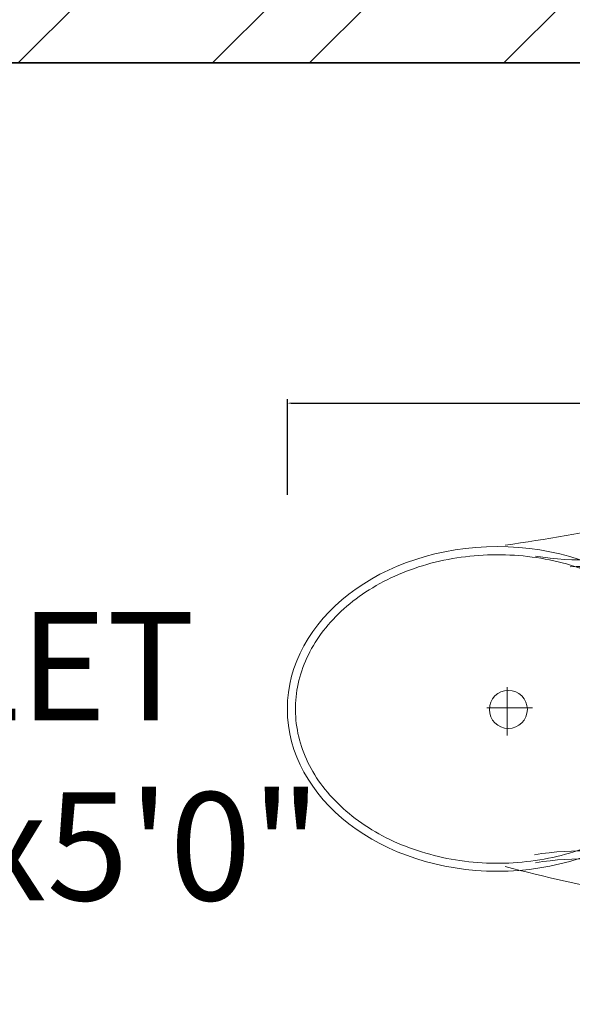
# Model space of a CAD drawing. Units: inches. Extents: x 2168 to 3056, y 1130 to 2629.
# Tile 36 of 42: x 2818 to 2843, y 2217 to 2263. Entities that reach past the tile are written whole.
import ezdxf

# ---------------------------------------------------------------- set-up
doc = ezdxf.new("R2010")
doc.units = ezdxf.units.IN
for name, color, linetype, lineweight in [('A-ANNO-DIMS', 2, 'Continuous', 18), ('A-AREA-IDEN', 7, 'Continuous', 18), ('A-FLOR-FIXT', 9, 'Continuous', 18), ('A-WALL', 7, 'Continuous', 35)]:
    doc.layers.add(name, color=color, linetype=linetype, lineweight=lineweight)
doc.layers.add('A-WALL-PATT', color=143, linetype='Continuous', lineweight=13, true_color=0x7aafdf)
doc.styles.get("Standard").update_dxf_attribs({"font": 'arial.ttf'})
doc.dimstyles.get("Standard").update_dxf_attribs({"dimtxt": 0.18, "dimasz": 0.18, "dimexe": 0.18, "dimexo": 0.0625, "dimgap": 0.09, "dimtad": 0, "dimtih": 1, "dimtoh": 1, "dimdec": 4, "dimzin": 0, "dimdsep": 46, "dimtxsty": 'Standard', "dimcen": 0.09, "dimadec": 0, "dimazin": 0, "dimtfac": 1, "dimtdec": 4, "dimtofl": 0, "dimtmove": 0, "dimatfit": 3, "dimfxl": 1, "dimtolj": 1, "dimtzin": 0, "dimarcsym": 0})

# ---------------------------------------------------------------- blocks, each defined once
blk = doc.blocks.new('A$C31115884')
for p, q in [((257.5, 466.4), (257.5, 523.2)), ((283.1, 497.7), (223.4, 497.7)), ((0, 200), (0, 0)), ((520, 200), (0, 200)), ((520, 0), (520, 200)), ((10, 190), (10, 10)), ((510, 190), (10, 190)), ((510, 10), (510, 190)), ((510, 54.5), (0, 54.5)), ((10, 10), (510, 10)), ((0, 0), (520, 0))]:
    blk.add_line(p, q)
blk.add_circle((255.6, 496.4), 23.6)
for centre, radius, start, end in [((2777.7, -204.6), 2807, 165.4549, 171.7133), ((3237, 905), 2807, 188.2867, 194.5451), ((-294.5, 403.3), 364.7, 324.2091, 9.3499), ((-294.5, 403.3), 374.7, 324.2091, 9.3499), ((805.8, 403.3), 364.7, 170.6501, 215.7909), ((139.5, 406.2), 293.5, 315.8436, 2.6563), ((805.8, 403.3), 374.7, 179.2036, 215.7909), ((383.6, 406.2), 293.5, 190.2774, 224.1564)]:
    blk.add_arc(centre, radius, start, end)
blk.add_ellipse((256.2, 509.9), major_axis=(0, -260.7), ratio=0.772727)
blk.add_open_spline([(256.2, 259.2), (263.1, 259.2), (270, 259.7), (287.8, 262.3), (298.7, 265.1), (319.9, 273.1), (330.2, 278.4), (350.1, 291.1), (359.7, 298.7), (377.7, 315.9), (386.2, 325.5), (401.7, 346.6), (408.8, 358.1), (421.3, 382.5), (426.8, 395.5), (435.9, 422.4), (439.5, 436.4), (444.8, 465.1), (446.5, 479.7), (447.9, 509.2), (447.6, 524), (445, 553.3), (442.7, 567.8), (436.3, 596), (432.1, 609.7), (421.9, 636), (416, 648.6), (402.5, 672.1), (395, 683), (378.6, 703), (369.8, 712.1), (351.1, 728), (341.3, 734.8), (320.9, 746.2), (310.4, 750.7), (288.9, 757.3), (278, 759.4), (256, 761), (245, 760.6), (223.1, 757.2), (212.3, 754.3), (191.1, 746.1), (180.8, 740.7), (160.9, 727.8), (151.4, 720.1), (133.5, 702.7), (125.1, 693), (109.6, 671.7), (102.6, 660.2), (90.2, 635.7), (84.9, 622.7), (76, 595.6), (72.4, 581.6), (67.2, 552.9), (65.6, 538.2), (64.4, 508.8), (64.8, 494), (67.5, 464.7), (69.9, 450.2), (76.6, 422), (80.8, 408.3), (91.1, 382.2), (97.2, 369.7), (110.8, 346.3), (118.4, 335.4), (134.8, 315.6), (143.7, 306.7), (162.4, 290.9), (172.3, 284.2), (192.8, 273), (203.3, 268.6), (224.8, 262.2), (235.8, 260.2), (249.9, 259.3), (253, 259.2), (256.2, 259.2)], degree=3, knots=[0, 0, 0, 0, 0.110105, 0.110105, 0.285049, 0.285049, 0.459994, 0.459994, 0.634938, 0.634938, 0.809882, 0.809882, 0.984827, 0.984827, 1.159771, 1.159771, 1.334715, 1.334715, 1.50966, 1.50966, 1.684604, 1.684604, 1.859549, 1.859549, 2.034493, 2.034493, 2.209437, 2.209437, 2.384382, 2.384382, 2.559326, 2.559326, 2.73427, 2.73427, 2.909215, 2.909215, 3.084159, 3.084159, 3.259103, 3.259103, 3.434048, 3.434048, 3.608992, 3.608992, 3.783936, 3.783936, 3.958881, 3.958881, 4.133825, 4.133825, 4.30877, 4.30877, 4.483714, 4.483714, 4.658658, 4.658658, 4.833603, 4.833603, 5.008547, 5.008547, 5.183491, 5.183491, 5.358436, 5.358436, 5.53338, 5.53338, 5.708324, 5.708324, 5.883269, 5.883269, 6.058213, 6.058213, 6.233158, 6.233158, 6.283185, 6.283185, 6.283185, 6.283185])
blk = doc.blocks.new('*D20')
at = {"layer": 'A-ANNO-DIMS', "color": 0, "lineweight": -2, "transparency": 16777216}
for p, q in [((2830.107, 2240.907), (2830.107, 2245.333)), ((2830.287, 2245.153), (2843.691, 2245.153)), ((2858.647, 2245.153), (2845.243, 2245.153)), ((2858.827, 2240.907), (2858.827, 2245.333))]:
    blk.add_line(p, q, dxfattribs=at)
at = {"layer": 'A-ANNO-DIMS', "color": 0, "transparency": 16777216}
for points in [[(2830.287, 2245.183), (2830.287, 2245.123), (2830.107, 2245.153)], [(2858.647, 2245.183), (2858.647, 2245.123), (2858.827, 2245.153)]]:
    blk.add_solid(points, dxfattribs=at)
at = {"layer": 'Defpoints', "color": 0, "transparency": 16777216}
for p in [(2830.107, 2245.153), (2830.107, 2240.845), (2858.827, 2240.845)]:
    blk.add_point(p, dxfattribs=at)
at = {"layer": 'A-ANNO-DIMS', "color": 0, "transparency": 16777216, "insert": (2844.467, 2245.153), "char_height": 0.18, "attachment_point": 5}
blk.add_mtext('\\A1;WC 29 TYP.', dxfattribs=at)

msp = doc.modelspace()

# ---------------------------------------------------------------- hatches: boundary and pattern name
at = {"layer": 'A-WALL-PATT'}
h = msp.add_hatch(dxfattribs=at)
h.set_pattern_fill('ANSI32', color=256)
h.paths.add_polyline_path([(2463.796, 2409.389), (2467.387, 2409.389), (2467.387, 2413.889), (2454.768, 2413.889), (2454.768, 2411.639), (2454.768, 2409.389), (2459.296, 2409.389), (2459.296, 2265.389), (2455.644, 2265.389), (2455.644, 2260.889), (2467.349, 2260.889), (2467.349, 2263.139), (2467.349, 2265.389), (2463.796, 2265.389)])
h.paths.add_polyline_path([(2431.596, 2413.889), (2409.647, 2413.889), (2409.647, 2409.389), (2431.596, 2409.389), (2431.596, 2411.639)])
h.paths.add_polyline_path([(2349.647, 2413.889), (2331.796, 2413.889), (2331.796, 2362.671), (2336.296, 2362.671), (2336.296, 2409.389), (2349.647, 2409.389), (2349.647, 2411.639)])
h.paths.add_polyline_path([(2634.149, 2411.639), (2634.149, 2413.889), (2562.293, 2413.889), (2562.293, 2409.389), (2595.796, 2409.389), (2595.796, 2280.309), (2595.826, 2280.309), (2595.826, 2265.389), (2499.91, 2265.389), (2499.91, 2260.889), (2550.796, 2260.889), (2550.796, 2117.308), (2555.296, 2117.308), (2555.296, 2168.08), (2571.93, 2168.08), (2571.93, 2176.889), (2559.796, 2176.889), (2559.796, 2256.389), (2640.796, 2256.389), (2640.796, 2176.889), (2626.428, 2176.889), (2626.428, 2168.08), (2645.296, 2168.08), (2645.296, 2116.637), (2649.796, 2116.637), (2649.796, 2260.889), (2691.251, 2260.889), (2691.251, 2263.139), (2691.251, 2265.389), (2670.655, 2265.389), (2670.655, 2265.365), (2600.296, 2265.365), (2600.296, 2280.258), (2600.296, 2409.389), (2634.149, 2409.389)])
h.paths.add_polyline_path([(2600.296, 2473.889), (2612.84, 2473.889), (2612.84, 2478.389), (2572.636, 2478.389), (2572.636, 2473.889), (2595.796, 2473.889), (2595.796, 2413.889), (2600.296, 2413.889)])
h.paths.add_polyline_path([(2535.796, 2473.889), (2548.636, 2473.889), (2548.636, 2478.389), (2531.396, 2478.389), (2531.396, 2413.889), (2521.6, 2413.889), (2521.6, 2409.389), (2539.239, 2409.389), (2539.239, 2411.639), (2539.239, 2413.889), (2535.796, 2413.889)])
h.paths.add_polyline_path([(2664.796, 2478.389), (2636.84, 2478.389), (2636.84, 2473.889), (2660.296, 2473.889), (2660.296, 2413.889), (2656.165, 2413.889), (2656.165, 2409.389), (2671.684, 2409.389), (2671.684, 2411.639), (2671.684, 2413.889), (2664.796, 2413.889)])
h.paths.add_polyline_path([(2705.942, 2413.889), (2695.684, 2413.889), (2695.684, 2409.389), (2705.942, 2409.389)])
h.paths.add_polyline_path([(2741.35, 2413.889), (2728.733, 2413.889), (2728.733, 2411.639), (2728.733, 2409.389), (2732.296, 2409.389), (2732.296, 2265.389), (2725.733, 2265.389), (2725.733, 2260.889), (2740.917, 2260.889), (2740.917, 2263.139), (2740.917, 2265.389), (2736.796, 2265.389), (2736.796, 2409.389), (2741.35, 2409.389)])
h.paths.add_polyline_path([(2785.655, 2413.889), (2764.546, 2413.889), (2764.486, 2409.389), (2785.655, 2409.389), (2785.655, 2411.639)])
h.paths.add_polyline_path([(2864.296, 2413.889), (2845.655, 2413.889), (2845.655, 2409.389), (2859.796, 2409.389), (2859.796, 2368.425), (2864.296, 2368.425)])
h.paths.add_polyline_path([(2864.296, 2308.425), (2862.046, 2308.425), (2859.796, 2308.425), (2859.796, 2265.389), (2774.483, 2265.389), (2774.483, 2263.139), (2774.483, 2260.889), (2781.796, 2260.889), (2781.796, 2226.654), (2786.296, 2226.654), (2786.296, 2260.889), (2859.796, 2260.889), (2859.796, 2241.352), (2864.296, 2241.352)])
h.paths.add_polyline_path([(2864.296, 2217.352), (2862.046, 2217.352), (2859.796, 2217.352), (2859.796, 2200.889), (2786.296, 2200.889), (2786.296, 2205.931), (2784.046, 2205.931), (2781.796, 2205.931), (2781.796, 2150.974), (2786.296, 2150.974), (2786.296, 2161.889), (2859.796, 2161.889), (2859.796, 2144.419), (2864.296, 2144.419)])
h.paths.add_polyline_path([(2859.796, 2196.389), (2859.796, 2166.389), (2786.296, 2166.389), (2786.296, 2196.389)], flags=16)
h.paths.add_polyline_path([(2864.296, 2108.419), (2862.046, 2108.419), (2859.796, 2108.419), (2859.796, 2080.889), (2786.296, 2080.889), (2786.296, 2111.993), (2781.796, 2111.993), (2781.796, 2080.889), (2649.796, 2080.889), (2649.796, 2086.036), (2647.546, 2086.036), (2645.296, 2086.036), (2645.296, 2071.739), (2649.796, 2071.739), (2649.796, 2076.389), (2781.796, 2076.389), (2781.796, 2041.792), (2786.296, 2041.792), (2786.296, 2076.389), (2859.796, 2076.389), (2859.796, 2058.577), (2864.296, 2058.577)])
h.paths.add_polyline_path([(2864.296, 2022.577), (2859.796, 2022.577), (2859.796, 1992.389), (2786.296, 1992.389), (2786.296, 1999.573), (2781.796, 1999.573), (2781.796, 1848.085), (2784.046, 1848.085), (2786.296, 1848.085), (2786.296, 1851.389), (2859.796, 1851.389), (2859.796, 1838.258), (2864.296, 1838.258)], flags=17)
h.paths.add_polyline_path([(2859.796, 1987.889), (2859.796, 1855.889), (2786.296, 1855.889), (2786.296, 1987.889)], flags=16)
h.paths.add_polyline_path([(2823.046, 1987.889), (2841.421, 1921.889), (2823.046, 1855.889)], flags=0)
h.paths.add_polyline_path([(2864.296, 1814.258), (2859.796, 1814.258), (2859.796, 1791.389), (2786.296, 1791.389), (2786.296, 1825.658), (2784.046, 1825.658), (2781.796, 1825.658), (2781.796, 1791.389), (2720.155, 1791.389), (2720.155, 1791.265), (2649.796, 1791.265), (2649.796, 1806.159), (2649.796, 2038.983), (2647.546, 2038.983), (2645.296, 2038.983), (2645.296, 1783.925), (2649.796, 1783.925), (2649.796, 1786.889), (2781.796, 1786.889), (2781.796, 1746.789), (2786.296, 1746.789), (2786.296, 1786.889), (2859.796, 1786.889), (2859.796, 1770.083), (2864.296, 1770.083)])
h.paths.add_polyline_path([(2864.296, 1734.083), (2862.046, 1734.083), (2859.796, 1734.083), (2859.796, 1705.889), (2786.296, 1705.889), (2786.296, 1714.166), (2781.796, 1714.166), (2781.796, 1660.527), (2786.296, 1660.527), (2786.296, 1666.889), (2859.796, 1666.889), (2859.796, 1648.342), (2864.296, 1648.342)])
h.paths.add_polyline_path([(2786.296, 1701.389), (2859.796, 1701.389), (2859.796, 1671.389), (2786.296, 1671.389)], flags=16)
h.paths.add_polyline_path([(2649.796, 1756.576), (2647.546, 1756.576), (2645.296, 1756.576), (2645.296, 1606.889), (2555.296, 1606.889), (2555.296, 1749.513), (2553.046, 1749.513), (2550.796, 1749.513), (2550.796, 1606.889), (2503.006, 1606.889), (2503.006, 1604.639), (2503.006, 1602.389), (2595.796, 1602.389), (2595.849, 1602.389), (2595.849, 1587.495), (2595.796, 1458.389), (2561.502, 1458.389), (2561.502, 1456.139), (2561.502, 1453.889), (2595.796, 1453.889), (2595.796, 1381.889), (2573.438, 1381.889), (2573.438, 1377.389), (2613.01, 1377.389), (2613.01, 1379.639), (2613.01, 1381.889), (2600.296, 1381.889), (2600.296, 1453.889), (2634.327, 1453.889), (2634.327, 1458.389), (2600.296, 1458.389), (2600.296, 1602.389), (2670.655, 1602.389), (2694.095, 1602.389), (2694.095, 1606.889), (2649.796, 1606.889)])
h.paths.add_polyline_path([(2736.796, 1602.389), (2741.562, 1602.389), (2741.562, 1606.889), (2726.203, 1606.889), (2726.203, 1604.639), (2726.203, 1602.389), (2732.296, 1602.389), (2732.296, 1458.389), (2727.899, 1458.389), (2727.899, 1453.889), (2740.821, 1453.889), (2740.821, 1456.139), (2740.821, 1458.389), (2736.796, 1458.389)])
h.paths.add_polyline_path([(2859.796, 1606.889), (2786.296, 1606.889), (2786.296, 1637.334), (2784.046, 1637.334), (2781.796, 1637.334), (2781.796, 1606.889), (2775.612, 1606.889), (2775.612, 1602.389), (2859.796, 1602.389)])
h.paths.add_polyline_path([(2864.296, 1624.342), (2862.046, 1624.342), (2859.796, 1624.342), (2859.796, 1570.39), (2864.296, 1570.39)])
h.paths.add_polyline_path([(2864.296, 1510.39), (2862.046, 1510.39), (2859.796, 1510.39), (2859.796, 1458.389), (2846.735, 1458.389), (2846.735, 1456.139), (2846.735, 1453.889), (2864.296, 1453.889)])
h.paths.add_polyline_path([(2786.735, 1458.389), (2765.444, 1458.389), (2765.444, 1453.889), (2786.735, 1453.889)])
h.paths.add_polyline_path([(2706.004, 1458.389), (2695.36, 1458.389), (2695.36, 1453.889), (2706.004, 1453.889), (2706.004, 1456.139)])
h.paths.add_polyline_path([(2671.36, 1456.139), (2671.36, 1458.389), (2655.986, 1458.389), (2655.986, 1456.139), (2655.986, 1453.889), (2660.296, 1453.889), (2660.296, 1381.889), (2637.01, 1381.889), (2637.01, 1377.389), (2664.796, 1377.389), (2664.796, 1453.889), (2671.36, 1453.889)], flags=17)
h.paths.add_polyline_path([(2539.829, 1458.389), (2520.237, 1458.389), (2520.237, 1453.889), (2531.296, 1453.889), (2531.296, 1377.389), (2546.449, 1377.389), (2546.449, 1379.639), (2546.449, 1381.889), (2535.796, 1381.889), (2535.796, 1453.889), (2539.829, 1453.889)], flags=17)
h.paths.add_polyline_path([(2496.237, 1458.389), (2489.13, 1458.389), (2489.13, 1453.889), (2496.237, 1453.889), (2496.237, 1456.139)])
h.paths.add_polyline_path([(2467.433, 1456.139), (2467.433, 1458.389), (2463.796, 1458.389), (2463.796, 1602.389), (2468.242, 1602.389), (2468.242, 1605.7), (2468.242, 1606.889), (2454.602, 1606.889), (2454.602, 1602.389), (2459.296, 1602.389), (2459.296, 1458.389), (2454.24, 1458.389), (2454.24, 1453.889), (2467.433, 1453.889)])
h.paths.add_polyline_path([(2431.601, 1456.139), (2431.601, 1458.389), (2411.386, 1458.389), (2411.386, 1453.889), (2431.601, 1453.889)])
h.paths.add_polyline_path([(2351.386, 1458.389), (2336.296, 1458.389), (2336.296, 1490.693), (2334.046, 1490.693), (2331.796, 1490.693), (2331.796, 1453.889), (2351.386, 1453.889), (2351.386, 1456.139)])
h.paths.add_polyline_path([(2336.296, 1629.705), (2331.796, 1629.705), (2331.796, 1552.317), (2336.296, 1552.317), (2336.296, 1602.389), (2406.655, 1602.389), (2423.472, 1602.389), (2423.472, 1606.889), (2418.796, 1606.889), (2418.796, 1643.678), (2416.546, 1643.678), (2414.296, 1643.678), (2414.296, 1606.889), (2336.296, 1606.889)])
h.paths.add_polyline_path([(2418.796, 1714.384), (2414.296, 1714.384), (2414.296, 1705.889), (2336.296, 1705.889), (2336.296, 1731.324), (2334.046, 1731.324), (2331.796, 1731.324), (2331.796, 1653.705), (2334.046, 1653.705), (2336.296, 1653.705), (2336.296, 1666.889), (2414.296, 1666.889), (2414.296, 1663.589), (2418.796, 1663.589)])
h.paths.add_polyline_path([(2336.296, 1701.389), (2414.296, 1701.389), (2414.296, 1671.389), (2336.296, 1671.389)], flags=16)
h.paths.add_polyline_path([(2555.296, 2040.059), (2550.796, 2040.059), (2550.796, 1791.389), (2550.561, 1791.205), (2480.202, 1791.205), (2418.796, 1791.389), (2418.796, 1825.448), (2416.546, 1825.448), (2414.296, 1825.448), (2414.296, 1791.389), (2336.296, 1791.389), (2336.296, 1806.409), (2331.796, 1806.409), (2331.796, 1767.324), (2336.296, 1767.324), (2336.296, 1786.889), (2414.296, 1786.889), (2414.296, 1745.457), (2418.796, 1745.457), (2418.796, 1786.889), (2550.796, 1786.889), (2550.796, 1783.011), (2555.296, 1783.011)])
h.paths.add_polyline_path([(2418.796, 1923.389), (2423.207, 1923.389), (2423.207, 1925.639), (2423.207, 1927.889), (2418.796, 1927.889), (2418.796, 2000.048), (2414.296, 2000.048), (2414.296, 1992.389), (2336.296, 1992.389), (2336.296, 1987.889), (2414.296, 1987.889), (2414.296, 1855.889), (2336.296, 1855.889), (2336.296, 1851.389), (2414.296, 1851.389), (2414.296, 1846.759), (2418.796, 1846.759)], flags=17)
h.paths.add_polyline_path([(2336.296, 2019.294), (2334.046, 2019.294), (2331.796, 2019.294), (2331.796, 1830.409), (2336.296, 1830.409)], flags=17)
h.paths.add_polyline_path([(2550.796, 1927.889), (2453.541, 1927.889), (2453.541, 1925.639), (2453.541, 1923.389), (2550.796, 1923.389)], flags=17)
h.paths.add_polyline_path([(2744.987, 1927.889), (2649.796, 1927.889), (2649.796, 1923.389), (2744.987, 1923.389), (2744.987, 1925.639)], flags=17)
h.paths.add_polyline_path([(2555.296, 2086.458), (2553.046, 2086.458), (2550.796, 2086.458), (2550.796, 2080.889), (2418.796, 2080.889), (2336.296, 2080.889), (2336.296, 2115.399), (2334.046, 2115.399), (2331.796, 2115.399), (2331.796, 2055.294), (2336.296, 2055.294), (2336.296, 2076.389), (2550.796, 2076.389), (2550.796, 2071.538), (2555.296, 2071.538)])
h.paths.add_polyline_path([(2418.796, 2121.389), (2414.296, 2121.389), (2414.296, 2080.889), (2418.796, 2080.889)])
h.paths.add_polyline_path([(2418.796, 2076.389), (2414.296, 2076.389), (2414.296, 2035.123), (2418.796, 2035.123)])
h.paths.add_polyline_path([(2422.868, 2263.139), (2422.868, 2265.389), (2406.655, 2265.389), (2406.655, 2265.359), (2336.296, 2265.359), (2336.296, 2280.252), (2336.296, 2302.671), (2334.046, 2302.671), (2331.796, 2302.671), (2331.796, 2246.853), (2336.296, 2246.853), (2336.296, 2260.889), (2414.296, 2260.889), (2414.296, 2223.996), (2418.796, 2223.996), (2418.796, 2260.889), (2422.868, 2260.889)])
h.paths.add_polyline_path([(2418.796, 2204.783), (2416.546, 2204.783), (2414.296, 2204.783), (2414.296, 2200.889), (2336.296, 2200.889), (2336.296, 2220.853), (2331.796, 2220.853), (2331.796, 2151.399), (2336.296, 2151.399), (2336.296, 2161.889), (2414.296, 2161.889), (2414.296, 2153.726), (2418.796, 2153.726)])
h.paths.add_polyline_path([(2414.296, 2196.389), (2414.296, 2166.389), (2336.296, 2166.389), (2336.296, 2196.389)], flags=16)
h.paths.add_polyline_path([(2375.296, 2181.389), (2336.296, 2166.389), (2336.296, 2196.389)], flags=0)
h.paths.add_polyline_path([(2809.595, 2172.34), (2838.804, 2172.34), (2838.804, 2190.997), (2809.595, 2190.997)], flags=8)
h.paths.add_polyline_path([(2849.75, 1919.585), (2849.75, 1952.672), (2831.093, 1952.672), (2831.093, 1919.585)], flags=8)
h.paths.add_polyline_path([(2808.875, 1901.967), (2808.875, 1937.85), (2790.149, 1937.85), (2790.149, 1901.967)], flags=8)
h.paths.add_polyline_path([(2806.285, 1671.896), (2835.493, 1671.896), (2835.493, 1690.553), (2806.285, 1690.553)], flags=8)
h.paths.add_polyline_path([(2353.186, 1676.549), (2382.395, 1676.549), (2382.395, 1695.207), (2353.186, 1695.207)], flags=8)
h.paths.add_polyline_path([(2360.083, 1832.308), (2389.241, 1832.308), (2389.241, 1850.966), (2360.083, 1850.966)], flags=25)
h.paths.add_polyline_path([(2354.822, 2167.823), (2384.031, 2167.823), (2384.031, 2186.481), (2354.822, 2186.481)], flags=8)

# ---------------------------------------------------------------- linework, layer by layer
at = {"layer": 'A-WALL'}
msp.add_line((2786.296, 2260.889), (2859.796, 2260.889), dxfattribs=at)

# ---------------------------------------------------------------- block references
at = {"layer": 'A-FLOR-FIXT', "xscale": 0.0372717239612423, "yscale": 0.0372717239612423, "zscale": 0.0372717239612423, "rotation": 89.99999999999999}
msp.add_blockref('A$C31115884', (2858.827, 2221.463), dxfattribs=at)

# ---------------------------------------------------------------- texts
at = {"layer": 'A-AREA-IDEN', "insert": (2802.88, 2235.492), "char_height": 5, "attachment_point": 1}
msp.add_mtext_dynamic_manual_height_columns('TOILET\\P6\'6"x5\'0"', width=169.35932, gutter_width=12.5, heights=[0], dxfattribs=at)

# ---------------------------------------------------------------- dimensions: what is measured, and where the dimension line sits
at = {"layer": 'A-ANNO-DIMS'}
dim = msp.add_linear_dim(base=(2830.107, 2245.153), p1=(2858.827, 2240.845), p2=(2830.107, 2240.845), angle=180, text='WC <> TYP.', dimstyle='Standard', override={"dimdec": 0, "dimlfac": 1, "dimrnd": 0, "dimzin": 0, "dimdsep": 46, "dimlunit": 2}, dxfattribs=at)
dim.commit()
dim.dimension.update_dxf_attribs({"geometry": '*D20', "text_midpoint": (2844.467, 2245.153)})

doc.saveas('drawing.dxf')
